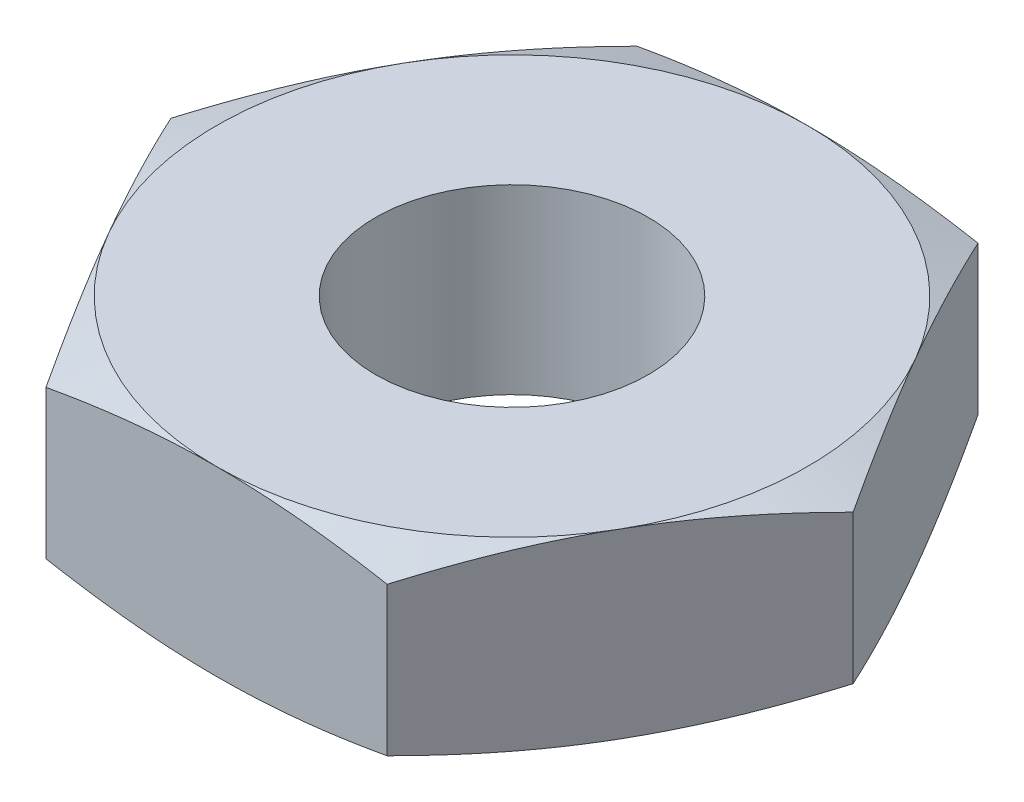
ISO-10303-21;
HEADER;
FILE_DESCRIPTION(('STEP AP214'),'2;1');
FILE_NAME('part.step','',(''),(''),'','','');
FILE_SCHEMA(('AUTOMOTIVE_DESIGN { 1 0 10303 214 1 1 1 1 }'));
ENDSEC;
DATA;
#1=APPLICATION_CONTEXT('core data for automotive mechanical design processes');
#2=APPLICATION_PROTOCOL_DEFINITION('international standard','automotive_design',2000,#1);
#3=PRODUCT_CONTEXT('',#1,'mechanical');
#4=PRODUCT('Part','Part','',(#3));
#5=PRODUCT_RELATED_PRODUCT_CATEGORY('part','',(#4));
#6=PRODUCT_DEFINITION_FORMATION('','',#4);
#7=PRODUCT_DEFINITION_CONTEXT('part definition',#1,'design');
#8=PRODUCT_DEFINITION('design','',#6,#7);
#9=PRODUCT_DEFINITION_SHAPE('','',#8);
#10=(LENGTH_UNIT() NAMED_UNIT(*) SI_UNIT(.MILLI.,.METRE.));
#11=(NAMED_UNIT(*) PLANE_ANGLE_UNIT() SI_UNIT($,.RADIAN.));
#12=(NAMED_UNIT(*) SI_UNIT($,.STERADIAN.) SOLID_ANGLE_UNIT());
#13=UNCERTAINTY_MEASURE_WITH_UNIT(LENGTH_MEASURE(1.E-05),#10,'distance_accuracy_value','');
#14=(GEOMETRIC_REPRESENTATION_CONTEXT(3) GLOBAL_UNCERTAINTY_ASSIGNED_CONTEXT((#13)) GLOBAL_UNIT_ASSIGNED_CONTEXT((#10,
#11,#12)) REPRESENTATION_CONTEXT('',''));
#15=CARTESIAN_POINT('',(0.,0.,0.));
#16=DIRECTION('',(0.,0.,1.));
#17=DIRECTION('',(1.,0.,0.));
#18=AXIS2_PLACEMENT_3D('',#15,#16,#17);
#19=CARTESIAN_POINT('',(0.,-4.,0.));
#20=DIRECTION('',(0.,1.,0.));
#21=DIRECTION('',(0.,0.,1.));
#22=AXIS2_PLACEMENT_3D('',#19,#20,#21);
#23=PLANE('',#22);
#24=CARTESIAN_POINT('',(0.,-4.,0.));
#25=DIRECTION('',(0.,1.,0.));
#26=DIRECTION('',(0.,0.,1.));
#27=AXIS2_PLACEMENT_3D('',#24,#25,#26);
#28=CIRCLE('',#27,6.);
#29=CARTESIAN_POINT('',(0.,-4.,6.));
#30=VERTEX_POINT('',#29);
#31=EDGE_CURVE('E260',#30,#30,#28,.T.);
#32=ORIENTED_EDGE('',*,*,#31,.T.);
#33=EDGE_LOOP('',(#32));
#34=FACE_BOUND('',#33,.T.);
#35=CARTESIAN_POINT('',(0.,-4.,0.));
#36=DIRECTION('',(0.,1.,0.));
#37=DIRECTION('',(0.,0.,1.));
#38=AXIS2_PLACEMENT_3D('',#35,#36,#37);
#39=CIRCLE('',#38,13.);
#40=CARTESIAN_POINT('',(1.35208313886344E-13,-4.,13.));
#41=VERTEX_POINT('',#40);
#42=CARTESIAN_POINT('',(11.2583302491977,-4.,6.49999999999994));
#43=VERTEX_POINT('',#42);
#44=EDGE_CURVE('E145',#41,#43,#39,.T.);
#45=ORIENTED_EDGE('',*,*,#44,.F.);
#46=CARTESIAN_POINT('',(0.,-4.,0.));
#47=DIRECTION('',(0.,1.,0.));
#48=DIRECTION('',(0.,0.,1.));
#49=AXIS2_PLACEMENT_3D('',#46,#47,#48);
#50=CIRCLE('',#49,13.);
#51=CARTESIAN_POINT('',(-11.2583302491977,-4.,6.50000000000009));
#52=VERTEX_POINT('',#51);
#53=EDGE_CURVE('E12',#41,#52,#50,.F.);
#54=ORIENTED_EDGE('',*,*,#53,.T.);
#55=CARTESIAN_POINT('',(-11.2583302491977,-4.,-6.49999999999993));
#56=VERTEX_POINT('',#55);
#57=EDGE_CURVE('E49',#52,#56,#50,.F.);
#58=ORIENTED_EDGE('',*,*,#57,.T.);
#59=CARTESIAN_POINT('',(0.,-4.,-13.));
#60=VERTEX_POINT('',#59);
#61=EDGE_CURVE('E456',#56,#60,#50,.F.);
#62=ORIENTED_EDGE('',*,*,#61,.T.);
#63=CARTESIAN_POINT('',(11.2583302491977,-4.,-6.50000000000002));
#64=VERTEX_POINT('',#63);
#65=EDGE_CURVE('E148',#60,#64,#50,.F.);
#66=ORIENTED_EDGE('',*,*,#65,.T.);
#67=EDGE_CURVE('E51',#64,#43,#50,.F.);
#68=ORIENTED_EDGE('',*,*,#67,.T.);
#69=EDGE_LOOP('',(#45,#54,#58,#62,#66,#68));
#70=FACE_BOUND('',#69,.T.);
#71=ADVANCED_FACE('F41',(#34,#70),#23,.F.);
#72=CARTESIAN_POINT('',(0.,4.,0.));
#73=DIRECTION('',(0.,1.,0.));
#74=DIRECTION('',(0.,0.,1.));
#75=AXIS2_PLACEMENT_3D('',#72,#73,#74);
#76=PLANE('',#75);
#77=CARTESIAN_POINT('',(0.,4.,0.));
#78=DIRECTION('',(0.,1.,0.));
#79=DIRECTION('',(0.,0.,1.));
#80=AXIS2_PLACEMENT_3D('',#77,#78,#79);
#81=CIRCLE('',#80,6.);
#82=CARTESIAN_POINT('',(0.,4.,6.));
#83=VERTEX_POINT('',#82);
#84=EDGE_CURVE('E251',#83,#83,#81,.T.);
#85=ORIENTED_EDGE('',*,*,#84,.F.);
#86=EDGE_LOOP('',(#85));
#87=FACE_BOUND('',#86,.T.);
#88=CARTESIAN_POINT('',(0.,4.,0.));
#89=DIRECTION('',(0.,1.,0.));
#90=DIRECTION('',(0.,0.,1.));
#91=AXIS2_PLACEMENT_3D('',#88,#89,#90);
#92=CIRCLE('',#91,13.);
#93=CARTESIAN_POINT('',(-11.2583302491976,4.,6.50000000000009));
#94=VERTEX_POINT('',#93);
#95=CARTESIAN_POINT('',(1.35308431126191E-13,4.,13.));
#96=VERTEX_POINT('',#95);
#97=EDGE_CURVE('E158',#94,#96,#92,.T.);
#98=ORIENTED_EDGE('',*,*,#97,.T.);
#99=CARTESIAN_POINT('',(11.2583302491978,4.,6.49999999999997));
#100=VERTEX_POINT('',#99);
#101=EDGE_CURVE('E156',#96,#100,#92,.T.);
#102=ORIENTED_EDGE('',*,*,#101,.T.);
#103=CARTESIAN_POINT('',(11.2583302491977,4.,-6.50000000000002));
#104=VERTEX_POINT('',#103);
#105=EDGE_CURVE('E302',#100,#104,#92,.T.);
#106=ORIENTED_EDGE('',*,*,#105,.T.);
#107=CARTESIAN_POINT('',(0.,4.,-13.));
#108=VERTEX_POINT('',#107);
#109=EDGE_CURVE('E308',#104,#108,#92,.T.);
#110=ORIENTED_EDGE('',*,*,#109,.T.);
#111=CARTESIAN_POINT('',(-11.2583302491977,4.,-6.49999999999993));
#112=VERTEX_POINT('',#111);
#113=EDGE_CURVE('E309',#108,#112,#92,.T.);
#114=ORIENTED_EDGE('',*,*,#113,.T.);
#115=EDGE_CURVE('E157',#112,#94,#92,.T.);
#116=ORIENTED_EDGE('',*,*,#115,.T.);
#117=EDGE_LOOP('',(#98,#102,#106,#110,#114,#116));
#118=FACE_BOUND('',#117,.T.);
#119=ADVANCED_FACE('F312',(#87,#118),#76,.T.);
#120=CARTESIAN_POINT('',(7.50555349946529,4.,12.9999999999999));
#121=DIRECTION('',(-0.866025403784441,0.,-0.499999999999995));
#122=DIRECTION('',(-0.499999999999995,0.,0.866025403784442));
#123=AXIS2_PLACEMENT_3D('',#120,#121,#122);
#124=PLANE('',#123);
#125=DIRECTION('',(0.,-1.,0.));
#126=VECTOR('',#125,1.);
#127=CARTESIAN_POINT('',(7.50555349946529,4.,12.9999999999999));
#128=LINE('',#127,#126);
#129=CARTESIAN_POINT('',(7.50555349946529,3.26801691446495,12.9999999999999));
#130=VERTEX_POINT('',#129);
#131=CARTESIAN_POINT('',(7.50555349946529,-3.26801691446495,12.9999999999999));
#132=VERTEX_POINT('',#131);
#133=EDGE_CURVE('E153',#130,#132,#128,.T.);
#134=ORIENTED_EDGE('',*,*,#133,.T.);
#135=CARTESIAN_POINT('',(7.50543802941145,-3.26797488631748,13.0001999999999));
#136=CARTESIAN_POINT('',(7.81626903778432,-3.3811479316258,12.4618249009302));
#137=CARTESIAN_POINT('',(8.12812500165726,-3.48409821469969,11.9216745268589));
#138=CARTESIAN_POINT('',(8.75386455582981,-3.66522307853089,10.8378618267266));
#139=CARTESIAN_POINT('',(9.06774953779601,-3.7433782740141,10.2941970902283));
#140=CARTESIAN_POINT('',(9.69406389084071,-3.86979198052381,9.20938880924519));
#141=CARTESIAN_POINT('',(10.0064789597828,-3.91832620674503,8.66827003678739));
#142=CARTESIAN_POINT('',(10.6320396475706,-3.98342422307978,7.58476714232116));
#143=CARTESIAN_POINT('',(10.9451849483842,-3.99999999999998,7.04238357116056));
#144=CARTESIAN_POINT('',(11.5714755500114,-3.99999999999998,5.95761642883936));
#145=CARTESIAN_POINT('',(11.884620850825,-3.98342422307978,5.41523285767877));
#146=CARTESIAN_POINT('',(12.5101815386128,-3.91832620674503,4.33172996321253));
#147=CARTESIAN_POINT('',(12.8225966075549,-3.8697919805238,3.79061119075473));
#148=CARTESIAN_POINT('',(13.4489109605996,-3.7433782740141,2.70580290977165));
#149=CARTESIAN_POINT('',(13.7627959425658,-3.66522307853089,2.16213817327336));
#150=CARTESIAN_POINT('',(14.3885354967383,-3.48409821469969,1.07832547314098));
#151=CARTESIAN_POINT('',(14.7003914606113,-3.3811479316258,0.538175099069677));
#152=CARTESIAN_POINT('',(15.0112224689841,-3.26797488631748,-0.000199999999997858));
#153=B_SPLINE_CURVE_WITH_KNOTS('',3,(#135,#136,#137,#138,#139,#140,#141,#142,#143,#144,#145,
#146,#147,#148,#149,#150,#151,#152),.UNSPECIFIED.,.F.,.F.,(4,2,2,2,2,2,2,2,4),(0.,
1.89583425179581,3.79314707118518,5.67251886941189,7.5511856255365,9.4298523816611,
11.3092241798878,13.2065369992772,15.102371251073),.UNSPECIFIED.);
#154=EDGE_CURVE('E64',#132,#43,#153,.T.);
#155=ORIENTED_EDGE('',*,*,#154,.T.);
#156=CARTESIAN_POINT('',(15.0111069989303,-3.26801691446495,0.));
#157=VERTEX_POINT('',#156);
#158=EDGE_CURVE('E132',#43,#157,#153,.T.);
#159=ORIENTED_EDGE('',*,*,#158,.T.);
#160=DIRECTION('',(0.,-1.,0.));
#161=VECTOR('',#160,1.);
#162=CARTESIAN_POINT('',(15.0111069989303,4.,0.));
#163=LINE('',#162,#161);
#164=CARTESIAN_POINT('',(15.0111069989303,3.26801691446495,0.));
#165=VERTEX_POINT('',#164);
#166=EDGE_CURVE('E271',#165,#157,#163,.T.);
#167=ORIENTED_EDGE('',*,*,#166,.F.);
#168=CARTESIAN_POINT('',(7.50543802941145,3.26797488631748,13.0001999999999));
#169=CARTESIAN_POINT('',(7.81626903778432,3.3811479316258,12.4618249009302));
#170=CARTESIAN_POINT('',(8.12812500165726,3.48409821469969,11.9216745268589));
#171=CARTESIAN_POINT('',(8.75386455582981,3.66522307853089,10.8378618267266));
#172=CARTESIAN_POINT('',(9.06774953779601,3.7433782740141,10.2941970902283));
#173=CARTESIAN_POINT('',(9.69406389084071,3.86979198052381,9.20938880924519));
#174=CARTESIAN_POINT('',(10.0064789597828,3.91832620674503,8.66827003678739));
#175=CARTESIAN_POINT('',(10.6320396475706,3.98342422307978,7.58476714232116));
#176=CARTESIAN_POINT('',(10.9451849483842,3.99999999999998,7.04238357116056));
#177=CARTESIAN_POINT('',(11.5714755500114,3.99999999999998,5.95761642883936));
#178=CARTESIAN_POINT('',(11.884620850825,3.98342422307978,5.41523285767877));
#179=CARTESIAN_POINT('',(12.5101815386128,3.91832620674503,4.33172996321253));
#180=CARTESIAN_POINT('',(12.8225966075549,3.8697919805238,3.79061119075473));
#181=CARTESIAN_POINT('',(13.4489109605996,3.7433782740141,2.70580290977165));
#182=CARTESIAN_POINT('',(13.7627959425658,3.66522307853089,2.16213817327336));
#183=CARTESIAN_POINT('',(14.3885354967383,3.48409821469969,1.07832547314098));
#184=CARTESIAN_POINT('',(14.7003914606113,3.3811479316258,0.538175099069677));
#185=CARTESIAN_POINT('',(15.0112224689841,3.26797488631748,-0.000199999999997858));
#186=B_SPLINE_CURVE_WITH_KNOTS('',3,(#168,#169,#170,#171,#172,#173,#174,#175,#176,#177,#178,
#179,#180,#181,#182,#183,#184,#185),.UNSPECIFIED.,.F.,.F.,(4,2,2,2,2,2,2,2,4),(0.,
1.89583425179581,3.79314707118518,5.67251886941189,7.5511856255365,9.4298523816611,
11.3092241798878,13.2065369992772,15.102371251073),.UNSPECIFIED.);
#187=EDGE_CURVE('E250',#100,#165,#186,.T.);
#188=ORIENTED_EDGE('',*,*,#187,.F.);
#189=EDGE_CURVE('E254',#130,#100,#186,.T.);
#190=ORIENTED_EDGE('',*,*,#189,.F.);
#191=EDGE_LOOP('',(#134,#155,#159,#167,#188,#190));
#192=FACE_BOUND('',#191,.T.);
#193=ADVANCED_FACE('F43',(#192),#124,.F.);
#194=CARTESIAN_POINT('',(15.0111069989303,4.,0.));
#195=DIRECTION('',(-0.866025403784438,0.,0.500000000000001));
#196=DIRECTION('',(0.500000000000001,0.,0.866025403784438));
#197=AXIS2_PLACEMENT_3D('',#194,#195,#196);
#198=PLANE('',#197);
#199=ORIENTED_EDGE('',*,*,#166,.T.);
#200=CARTESIAN_POINT('',(15.0112224689841,-3.26797488631748,0.000200000000000042));
#201=CARTESIAN_POINT('',(14.7003914606112,-3.38114793162581,-0.53817509906968));
#202=CARTESIAN_POINT('',(14.3885354967383,-3.48409821469969,-1.07832547314099));
#203=CARTESIAN_POINT('',(13.7627959425657,-3.6652230785309,-2.16213817327337));
#204=CARTESIAN_POINT('',(13.4489109605995,-3.74337827401411,-2.70580290977167));
#205=CARTESIAN_POINT('',(12.8225966075548,-3.86979198052382,-3.79061119075476));
#206=CARTESIAN_POINT('',(12.5101815386127,-3.91832620674505,-4.33172996321257));
#207=CARTESIAN_POINT('',(11.8846208508249,-3.9834242230798,-5.41523285767881));
#208=CARTESIAN_POINT('',(11.5714755500113,-4.,-5.95761642883941));
#209=CARTESIAN_POINT('',(10.9451849483841,-4.,-7.04238357116062));
#210=CARTESIAN_POINT('',(10.6320396475705,-3.9834242230798,-7.58476714232122));
#211=CARTESIAN_POINT('',(10.0064789597827,-3.91832620674505,-8.66827003678746));
#212=CARTESIAN_POINT('',(9.69406389084059,-3.86979198052382,-9.20938880924526));
#213=CARTESIAN_POINT('',(9.06774953779586,-3.74337827401411,-10.2941970902284));
#214=CARTESIAN_POINT('',(8.75386455582966,-3.6652230785309,-10.8378618267267));
#215=CARTESIAN_POINT('',(8.12812500165709,-3.48409821469969,-11.921674526859));
#216=CARTESIAN_POINT('',(7.81626903778414,-3.38114793162581,-12.4618249009303));
#217=CARTESIAN_POINT('',(7.50543802941127,-3.26797488631748,-13.0002));
#218=B_SPLINE_CURVE_WITH_KNOTS('',3,(#200,#201,#202,#203,#204,#205,#206,#207,#208,#209,#210,
#211,#212,#213,#214,#215,#216,#217),.UNSPECIFIED.,.F.,.F.,(4,2,2,2,2,2,2,2,4),(0.,
1.89583425179583,3.79314707118523,5.67251886941196,7.55118562553659,9.42985238166122,
11.309224179888,13.2065369992774,15.1023712510732),.UNSPECIFIED.);
#219=EDGE_CURVE('E138',#157,#64,#218,.T.);
#220=ORIENTED_EDGE('',*,*,#219,.T.);
#221=CARTESIAN_POINT('',(7.50555349946511,-3.26801691446495,-13.));
#222=VERTEX_POINT('',#221);
#223=EDGE_CURVE('E170',#64,#222,#218,.T.);
#224=ORIENTED_EDGE('',*,*,#223,.T.);
#225=DIRECTION('',(0.,-1.,0.));
#226=VECTOR('',#225,1.);
#227=CARTESIAN_POINT('',(7.50555349946511,4.,-13.));
#228=LINE('',#227,#226);
#229=CARTESIAN_POINT('',(7.50555349946511,3.26801691446495,-13.));
#230=VERTEX_POINT('',#229);
#231=EDGE_CURVE('E266',#230,#222,#228,.T.);
#232=ORIENTED_EDGE('',*,*,#231,.F.);
#233=CARTESIAN_POINT('',(15.0112224689841,3.26797488631748,0.000200000000000042));
#234=CARTESIAN_POINT('',(14.7003914606112,3.38114793162581,-0.53817509906968));
#235=CARTESIAN_POINT('',(14.3885354967383,3.48409821469969,-1.07832547314099));
#236=CARTESIAN_POINT('',(13.7627959425657,3.6652230785309,-2.16213817327337));
#237=CARTESIAN_POINT('',(13.4489109605995,3.74337827401411,-2.70580290977167));
#238=CARTESIAN_POINT('',(12.8225966075548,3.86979198052382,-3.79061119075476));
#239=CARTESIAN_POINT('',(12.5101815386127,3.91832620674505,-4.33172996321257));
#240=CARTESIAN_POINT('',(11.8846208508249,3.9834242230798,-5.41523285767881));
#241=CARTESIAN_POINT('',(11.5714755500113,4.,-5.95761642883941));
#242=CARTESIAN_POINT('',(10.9451849483841,4.,-7.04238357116062));
#243=CARTESIAN_POINT('',(10.6320396475705,3.9834242230798,-7.58476714232122));
#244=CARTESIAN_POINT('',(10.0064789597827,3.91832620674505,-8.66827003678746));
#245=CARTESIAN_POINT('',(9.69406389084059,3.86979198052382,-9.20938880924526));
#246=CARTESIAN_POINT('',(9.06774953779586,3.74337827401411,-10.2941970902284));
#247=CARTESIAN_POINT('',(8.75386455582966,3.6652230785309,-10.8378618267267));
#248=CARTESIAN_POINT('',(8.12812500165709,3.48409821469969,-11.921674526859));
#249=CARTESIAN_POINT('',(7.81626903778414,3.38114793162581,-12.4618249009303));
#250=CARTESIAN_POINT('',(7.50543802941127,3.26797488631748,-13.0002));
#251=B_SPLINE_CURVE_WITH_KNOTS('',3,(#233,#234,#235,#236,#237,#238,#239,#240,#241,#242,#243,
#244,#245,#246,#247,#248,#249,#250),.UNSPECIFIED.,.F.,.F.,(4,2,2,2,2,2,2,2,4),(0.,
1.89583425179583,3.79314707118523,5.67251886941196,7.55118562553659,9.42985238166122,
11.309224179888,13.2065369992774,15.1023712510732),.UNSPECIFIED.);
#252=EDGE_CURVE('E239',#104,#230,#251,.T.);
#253=ORIENTED_EDGE('',*,*,#252,.F.);
#254=EDGE_CURVE('E246',#165,#104,#251,.T.);
#255=ORIENTED_EDGE('',*,*,#254,.F.);
#256=EDGE_LOOP('',(#199,#220,#224,#232,#253,#255));
#257=FACE_BOUND('',#256,.T.);
#258=ADVANCED_FACE('F218',(#257),#198,.F.);
#259=CARTESIAN_POINT('',(7.50555349946511,4.,-13.));
#260=DIRECTION('',(0.,0.,1.));
#261=DIRECTION('',(1.,0.,0.));
#262=AXIS2_PLACEMENT_3D('',#259,#260,#261);
#263=PLANE('',#262);
#264=ORIENTED_EDGE('',*,*,#231,.T.);
#265=CARTESIAN_POINT('',(24.5155545956959,1.36823250554055,-13.0000000000001));
#266=CARTESIAN_POINT('',(24.0405240295999,1.21549334301211,-13.0000000000001));
#267=CARTESIAN_POINT('',(23.5652140208819,1.063618435089,-13.0000000000001));
#268=CARTESIAN_POINT('',(22.6139411221326,0.761910318310484,-13.0000000000001));
#269=CARTESIAN_POINT('',(22.1379782252003,0.612077131221862,-13.0000000000001));
#270=CARTESIAN_POINT('',(21.185215660392,0.314737702143928,-13.0000000000001));
#271=CARTESIAN_POINT('',(20.7084158378096,0.167231955324839,-13.0000000000001));
#272=CARTESIAN_POINT('',(19.7539723799837,-0.125022680870063,-13.0000000000001));
#273=CARTESIAN_POINT('',(19.2763287466556,-0.269771576494738,-13.0000000000001));
#274=CARTESIAN_POINT('',(18.3122096400441,-0.558389376293444,-13.0000000000001));
#275=CARTESIAN_POINT('',(17.8257180947263,-0.70220466785382,-13.0000000000001));
#276=CARTESIAN_POINT('',(16.8515839809399,-0.985880989376546,-13.0000000000001));
#277=CARTESIAN_POINT('',(16.3639414177948,-1.12574203758895,-13.0000000000001));
#278=CARTESIAN_POINT('',(15.3873473631516,-1.40075431206701,-13.0000000000001));
#279=CARTESIAN_POINT('',(14.8983959224935,-1.53590571848869,-13.));
#280=CARTESIAN_POINT('',(13.9189691583564,-1.80058323746787,-13.));
#281=CARTESIAN_POINT('',(13.428493836208,-1.93010935493618,-13.));
#282=CARTESIAN_POINT('',(12.4681215109835,-2.17667647391496,-13.));
#283=CARTESIAN_POINT('',(11.9983017482554,-2.29401734212416,-13.));
#284=CARTESIAN_POINT('',(11.0568829216087,-2.52135287481595,-13.));
#285=CARTESIAN_POINT('',(10.5852838557062,-2.63134753110473,-13.));
#286=CARTESIAN_POINT('',(9.64003084776995,-2.84258990322838,-13.));
#287=CARTESIAN_POINT('',(9.16637658007017,-2.9438361753631,-13.));
#288=CARTESIAN_POINT('',(8.21697677002227,-3.13589877665886,-13.));
#289=CARTESIAN_POINT('',(7.74123122545284,-3.22671509473869,-13.));
#290=CARTESIAN_POINT('',(6.31910363449161,-3.47919521660132,-13.));
#291=CARTESIAN_POINT('',(5.36932395191108,-3.62285615701864,-13.));
#292=CARTESIAN_POINT('',(3.93925896632588,-3.79026925410424,-13.));
#293=CARTESIAN_POINT('',(3.46174282400493,-3.83805703289572,-13.));
#294=CARTESIAN_POINT('',(2.50523859716394,-3.91592711867877,-13.));
#295=CARTESIAN_POINT('',(2.02625050436415,-3.9460093258922,-13.));
#296=CARTESIAN_POINT('',(1.00608586276806,-3.98987319438264,-13.));
#297=CARTESIAN_POINT('',(0.464795352583161,-4.00107614649847,-13.));
#298=CARTESIAN_POINT('',(-0.617736217142298,-3.99876013196134,-13.));
#299=CARTESIAN_POINT('',(-1.15897727593229,-3.98524083761707,-13.));
#300=CARTESIAN_POINT('',(-2.24052002292679,-3.93421249506995,-13.));
#301=CARTESIAN_POINT('',(-2.78082126229037,-3.89669409003737,-13.));
#302=CARTESIAN_POINT('',(-3.85941505627078,-3.79955682519537,-13.));
#303=CARTESIAN_POINT('',(-4.39770756186364,-3.73993742951957,-13.));
#304=CARTESIAN_POINT('',(-5.47704146456944,-3.60052693841533,-13.));
#305=CARTESIAN_POINT('',(-6.01805758084636,-3.5205426199044,-13.));
#306=CARTESIAN_POINT('',(-7.09728629812356,-3.34363373953174,-13.));
#307=CARTESIAN_POINT('',(-7.63549887790093,-3.24670904962198,-13.));
#308=CARTESIAN_POINT('',(-8.70920964168745,-3.03872213356502,-13.));
#309=CARTESIAN_POINT('',(-9.24470758968157,-2.92765869936841,-13.));
#310=CARTESIAN_POINT('',(-10.3131373904122,-2.6938904888945,-13.));
#311=CARTESIAN_POINT('',(-10.8460692509991,-2.57118574825494,-13.));
#312=CARTESIAN_POINT('',(-11.9378787322153,-2.30946863118862,-13.));
#313=CARTESIAN_POINT('',(-12.496631109914,-2.16993626646767,-13.));
#314=CARTESIAN_POINT('',(-13.61191651028,-1.88230159824707,-13.));
#315=CARTESIAN_POINT('',(-14.1684495289799,-1.73419927943467,-13.));
#316=CARTESIAN_POINT('',(-15.2795521826457,-1.43104180462645,-12.9999999999999));
#317=CARTESIAN_POINT('',(-15.83412201007,-1.27598735175158,-12.9999999999999));
#318=CARTESIAN_POINT('',(-16.941638337672,-0.960181887271385,-12.9999999999999));
#319=CARTESIAN_POINT('',(-17.4945848238111,-0.799430826558432,-12.9999999999999));
#320=CARTESIAN_POINT('',(-18.5881502472213,-0.476472370913964,-12.9999999999999));
#321=CARTESIAN_POINT('',(-19.128796391371,-0.314356915140173,-12.9999999999999));
#322=CARTESIAN_POINT('',(-20.2089506297819,0.0136235671370092,-12.9999999999999));
#323=CARTESIAN_POINT('',(-20.748458720098,0.179488606615906,-12.9999999999999));
#324=CARTESIAN_POINT('',(-21.8263834446703,0.514319692132321,-12.9999999999999));
#325=CARTESIAN_POINT('',(-22.3648002881825,0.683285065514164,-12.9999999999999));
#326=CARTESIAN_POINT('',(-23.4407814868745,1.02387855364092,-12.9999999999999));
#327=CARTESIAN_POINT('',(-23.9783458563606,1.19550662316754,-12.9999999999999));
#328=CARTESIAN_POINT('',(-24.515554595696,1.36823250554055,-12.9999999999999));
#329=B_SPLINE_CURVE_WITH_KNOTS('',3,(#265,#266,#267,#268,#269,#270,#271,#272,#273,#274,#275,
#276,#277,#278,#279,#280,#281,#282,#283,#284,#285,#286,#287,#288,#289,#290,#291,#292,#293,#294,
#295,#296,#297,#298,#299,#300,#301,#302,#303,#304,#305,#306,#307,#308,#309,#310,#311,#312,#313,
#314,#315,#316,#317,#318,#319,#320,#321,#322,#323,#324,#325,#326,#327,#328),.UNSPECIFIED.,.F.,
.F.,(4,2,2,2,2,2,2,2,2,2,2,2,2,2,2,2,2,2,2,2,2,2,2,2,2,2,2,2,2,2,2,4),(0.,1.49694813967669,
2.99391222584255,4.49119061440192,5.98846560872694,7.51036210879345,9.03225158369156,
10.5540827783197,12.0759126443824,13.5286166449153,14.9813222657356,16.4342671629383,
17.8872136037934,20.7669364113332,22.2063696578436,23.6458110160719,25.2694632279234,
26.893136961305,28.5174441225877,30.1417906698226,31.7821640738609,33.4225498776076,
35.063075934178,36.7035969687382,38.4312458729983,40.1588978643094,41.8863755177535,
43.6138680665518,45.3071379597887,47.0004137135154,48.6933263352441,50.3862102390845),.UNSPECIFIED.);
#330=EDGE_CURVE('E211',#222,#60,#329,.T.);
#331=ORIENTED_EDGE('',*,*,#330,.T.);
#332=CARTESIAN_POINT('',(-7.5055534994652,-3.26801691446495,-13.));
#333=VERTEX_POINT('',#332);
#334=EDGE_CURVE('E210',#60,#333,#329,.T.);
#335=ORIENTED_EDGE('',*,*,#334,.T.);
#336=DIRECTION('',(0.,-1.,0.));
#337=VECTOR('',#336,1.);
#338=CARTESIAN_POINT('',(-7.5055534994652,4.,-13.));
#339=LINE('',#338,#337);
#340=CARTESIAN_POINT('',(-7.5055534994652,3.26801691446495,-13.));
#341=VERTEX_POINT('',#340);
#342=EDGE_CURVE('E269',#341,#333,#339,.T.);
#343=ORIENTED_EDGE('',*,*,#342,.F.);
#344=CARTESIAN_POINT('',(24.5155545956959,-1.36823250554055,-13.0000000000001));
#345=CARTESIAN_POINT('',(24.0405240295999,-1.21549334301211,-13.0000000000001));
#346=CARTESIAN_POINT('',(23.5652140208819,-1.063618435089,-13.0000000000001));
#347=CARTESIAN_POINT('',(22.6139411221326,-0.761910318310484,-13.0000000000001));
#348=CARTESIAN_POINT('',(22.1379782252003,-0.612077131221862,-13.0000000000001));
#349=CARTESIAN_POINT('',(21.185215660392,-0.314737702143928,-13.0000000000001));
#350=CARTESIAN_POINT('',(20.7084158378096,-0.167231955324839,-13.0000000000001));
#351=CARTESIAN_POINT('',(19.7539723799837,0.125022680870063,-13.0000000000001));
#352=CARTESIAN_POINT('',(19.2763287466556,0.269771576494738,-13.0000000000001));
#353=CARTESIAN_POINT('',(18.3122096400441,0.558389376293444,-13.0000000000001));
#354=CARTESIAN_POINT('',(17.8257180947263,0.70220466785382,-13.0000000000001));
#355=CARTESIAN_POINT('',(16.8515839809399,0.985880989376546,-13.0000000000001));
#356=CARTESIAN_POINT('',(16.3639414177948,1.12574203758895,-13.0000000000001));
#357=CARTESIAN_POINT('',(15.3873473631516,1.40075431206701,-13.0000000000001));
#358=CARTESIAN_POINT('',(14.8983959224935,1.53590571848869,-13.));
#359=CARTESIAN_POINT('',(13.9189691583564,1.80058323746787,-13.));
#360=CARTESIAN_POINT('',(13.428493836208,1.93010935493618,-13.));
#361=CARTESIAN_POINT('',(12.4681215109835,2.17667647391496,-13.));
#362=CARTESIAN_POINT('',(11.9983017482554,2.29401734212416,-13.));
#363=CARTESIAN_POINT('',(11.0568829216087,2.52135287481595,-13.));
#364=CARTESIAN_POINT('',(10.5852838557062,2.63134753110473,-13.));
#365=CARTESIAN_POINT('',(9.64003084776995,2.84258990322838,-13.));
#366=CARTESIAN_POINT('',(9.16637658007017,2.9438361753631,-13.));
#367=CARTESIAN_POINT('',(8.21697677002227,3.13589877665886,-13.));
#368=CARTESIAN_POINT('',(7.74123122545284,3.22671509473869,-13.));
#369=CARTESIAN_POINT('',(6.31910363449161,3.47919521660132,-13.));
#370=CARTESIAN_POINT('',(5.36932395191108,3.62285615701864,-13.));
#371=CARTESIAN_POINT('',(3.93925896632588,3.79026925410424,-13.));
#372=CARTESIAN_POINT('',(3.46174282400493,3.83805703289572,-13.));
#373=CARTESIAN_POINT('',(2.50523859716394,3.91592711867877,-13.));
#374=CARTESIAN_POINT('',(2.02625050436415,3.9460093258922,-13.));
#375=CARTESIAN_POINT('',(1.00608586276806,3.98987319438264,-13.));
#376=CARTESIAN_POINT('',(0.464795352583161,4.00107614649847,-13.));
#377=CARTESIAN_POINT('',(-0.617736217142298,3.99876013196134,-13.));
#378=CARTESIAN_POINT('',(-1.15897727593229,3.98524083761707,-13.));
#379=CARTESIAN_POINT('',(-2.24052002292679,3.93421249506995,-13.));
#380=CARTESIAN_POINT('',(-2.78082126229037,3.89669409003737,-13.));
#381=CARTESIAN_POINT('',(-3.85941505627078,3.79955682519537,-13.));
#382=CARTESIAN_POINT('',(-4.39770756186364,3.73993742951957,-13.));
#383=CARTESIAN_POINT('',(-5.47704146456944,3.60052693841533,-13.));
#384=CARTESIAN_POINT('',(-6.01805758084636,3.5205426199044,-13.));
#385=CARTESIAN_POINT('',(-7.09728629812356,3.34363373953174,-13.));
#386=CARTESIAN_POINT('',(-7.63549887790093,3.24670904962198,-13.));
#387=CARTESIAN_POINT('',(-8.70920964168745,3.03872213356502,-13.));
#388=CARTESIAN_POINT('',(-9.24470758968157,2.92765869936841,-13.));
#389=CARTESIAN_POINT('',(-10.3131373904122,2.6938904888945,-13.));
#390=CARTESIAN_POINT('',(-10.8460692509991,2.57118574825494,-13.));
#391=CARTESIAN_POINT('',(-11.9378787322153,2.30946863118862,-13.));
#392=CARTESIAN_POINT('',(-12.496631109914,2.16993626646767,-13.));
#393=CARTESIAN_POINT('',(-13.61191651028,1.88230159824707,-13.));
#394=CARTESIAN_POINT('',(-14.1684495289799,1.73419927943467,-13.));
#395=CARTESIAN_POINT('',(-15.2795521826457,1.43104180462645,-12.9999999999999));
#396=CARTESIAN_POINT('',(-15.83412201007,1.27598735175158,-12.9999999999999));
#397=CARTESIAN_POINT('',(-16.941638337672,0.960181887271385,-12.9999999999999));
#398=CARTESIAN_POINT('',(-17.4945848238111,0.799430826558432,-12.9999999999999));
#399=CARTESIAN_POINT('',(-18.5881502472213,0.476472370913964,-12.9999999999999));
#400=CARTESIAN_POINT('',(-19.128796391371,0.314356915140173,-12.9999999999999));
#401=CARTESIAN_POINT('',(-20.2089506297819,-0.0136235671370092,-12.9999999999999));
#402=CARTESIAN_POINT('',(-20.748458720098,-0.179488606615906,-12.9999999999999));
#403=CARTESIAN_POINT('',(-21.8263834446703,-0.514319692132321,-12.9999999999999));
#404=CARTESIAN_POINT('',(-22.3648002881825,-0.683285065514164,-12.9999999999999));
#405=CARTESIAN_POINT('',(-23.4407814868745,-1.02387855364092,-12.9999999999999));
#406=CARTESIAN_POINT('',(-23.9783458563606,-1.19550662316754,-12.9999999999999));
#407=CARTESIAN_POINT('',(-24.515554595696,-1.36823250554055,-12.9999999999999));
#408=B_SPLINE_CURVE_WITH_KNOTS('',3,(#344,#345,#346,#347,#348,#349,#350,#351,#352,#353,#354,
#355,#356,#357,#358,#359,#360,#361,#362,#363,#364,#365,#366,#367,#368,#369,#370,#371,#372,#373,
#374,#375,#376,#377,#378,#379,#380,#381,#382,#383,#384,#385,#386,#387,#388,#389,#390,#391,#392,
#393,#394,#395,#396,#397,#398,#399,#400,#401,#402,#403,#404,#405,#406,#407),.UNSPECIFIED.,.F.,
.F.,(4,2,2,2,2,2,2,2,2,2,2,2,2,2,2,2,2,2,2,2,2,2,2,2,2,2,2,2,2,2,2,4),(0.,1.49694813967669,
2.99391222584255,4.49119061440192,5.98846560872694,7.51036210879345,9.03225158369156,
10.5540827783197,12.0759126443824,13.5286166449153,14.9813222657356,16.4342671629383,
17.8872136037934,20.7669364113332,22.2063696578436,23.6458110160719,25.2694632279234,
26.893136961305,28.5174441225877,30.1417906698226,31.7821640738609,33.4225498776076,
35.063075934178,36.7035969687382,38.4312458729983,40.1588978643094,41.8863755177535,
43.6138680665518,45.3071379597887,47.0004137135154,48.6933263352441,50.3862102390845),.UNSPECIFIED.);
#409=EDGE_CURVE('E228',#108,#341,#408,.T.);
#410=ORIENTED_EDGE('',*,*,#409,.F.);
#411=EDGE_CURVE('E231',#230,#108,#408,.T.);
#412=ORIENTED_EDGE('',*,*,#411,.F.);
#413=EDGE_LOOP('',(#264,#331,#335,#343,#410,#412));
#414=FACE_BOUND('',#413,.T.);
#415=ADVANCED_FACE('F217',(#414),#263,.F.);
#416=CARTESIAN_POINT('',(-7.5055534994652,4.,-13.));
#417=DIRECTION('',(0.866025403784442,0.,0.499999999999995));
#418=DIRECTION('',(0.499999999999995,0.,-0.866025403784442));
#419=AXIS2_PLACEMENT_3D('',#416,#417,#418);
#420=PLANE('',#419);
#421=ORIENTED_EDGE('',*,*,#342,.T.);
#422=CARTESIAN_POINT('',(-7.50543802941136,-3.26797488631748,-13.0002));
#423=CARTESIAN_POINT('',(-7.81626903778423,-3.38114793162581,-12.4618249009303));
#424=CARTESIAN_POINT('',(-8.12812500165717,-3.48409821469969,-11.921674526859));
#425=CARTESIAN_POINT('',(-8.75386455582973,-3.6652230785309,-10.8378618267266));
#426=CARTESIAN_POINT('',(-9.06774953779593,-3.74337827401411,-10.2941970902283));
#427=CARTESIAN_POINT('',(-9.69406389084065,-3.86979198052382,-9.2093888092452));
#428=CARTESIAN_POINT('',(-10.0064789597827,-3.91832620674505,-8.66827003678739));
#429=CARTESIAN_POINT('',(-10.6320396475705,-3.9834242230798,-7.58476714232115));
#430=CARTESIAN_POINT('',(-10.9451849483841,-4.,-7.04238357116054));
#431=CARTESIAN_POINT('',(-11.5714755500113,-4.,-5.95761642883933));
#432=CARTESIAN_POINT('',(-11.8846208508249,-3.9834242230798,-5.41523285767873));
#433=CARTESIAN_POINT('',(-12.5101815386128,-3.91832620674505,-4.33172996321248));
#434=CARTESIAN_POINT('',(-12.8225966075548,-3.86979198052382,-3.79061119075468));
#435=CARTESIAN_POINT('',(-13.4489109605995,-3.74337827401411,-2.70580290977158));
#436=CARTESIAN_POINT('',(-13.7627959425657,-3.6652230785309,-2.16213817327328));
#437=CARTESIAN_POINT('',(-14.3885354967383,-3.4840982146997,-1.07832547314089));
#438=CARTESIAN_POINT('',(-14.7003914606112,-3.38114793162581,-0.538175099069577));
#439=CARTESIAN_POINT('',(-15.0112224689841,-3.26797488631748,0.000200000000103726));
#440=B_SPLINE_CURVE_WITH_KNOTS('',3,(#422,#423,#424,#425,#426,#427,#428,#429,#430,#431,#432,
#433,#434,#435,#436,#437,#438,#439),.UNSPECIFIED.,.F.,.F.,(4,2,2,2,2,2,2,2,4),(0.,
1.89583425179583,3.79314707118523,5.67251886941196,7.55118562553659,9.42985238166122,
11.3092241798879,13.2065369992773,15.1023712510732),.UNSPECIFIED.);
#441=EDGE_CURVE('E213',#333,#56,#440,.T.);
#442=ORIENTED_EDGE('',*,*,#441,.T.);
#443=CARTESIAN_POINT('',(-15.0111069989303,-3.26801691446495,1.04808663662242E-13));
#444=VERTEX_POINT('',#443);
#445=EDGE_CURVE('E203',#56,#444,#440,.T.);
#446=ORIENTED_EDGE('',*,*,#445,.T.);
#447=DIRECTION('',(0.,-1.,0.));
#448=VECTOR('',#447,1.);
#449=CARTESIAN_POINT('',(-15.0111069989303,4.,1.04821999924285E-13));
#450=LINE('',#449,#448);
#451=CARTESIAN_POINT('',(-15.0111069989303,3.26801691446495,1.04808663662242E-13));
#452=VERTEX_POINT('',#451);
#453=EDGE_CURVE('E261',#452,#444,#450,.T.);
#454=ORIENTED_EDGE('',*,*,#453,.F.);
#455=CARTESIAN_POINT('',(-7.50543802941136,3.26797488631748,-13.0002));
#456=CARTESIAN_POINT('',(-7.81626903778423,3.38114793162581,-12.4618249009303));
#457=CARTESIAN_POINT('',(-8.12812500165717,3.48409821469969,-11.921674526859));
#458=CARTESIAN_POINT('',(-8.75386455582973,3.6652230785309,-10.8378618267266));
#459=CARTESIAN_POINT('',(-9.06774953779593,3.74337827401411,-10.2941970902283));
#460=CARTESIAN_POINT('',(-9.69406389084065,3.86979198052382,-9.2093888092452));
#461=CARTESIAN_POINT('',(-10.0064789597827,3.91832620674505,-8.66827003678739));
#462=CARTESIAN_POINT('',(-10.6320396475705,3.9834242230798,-7.58476714232115));
#463=CARTESIAN_POINT('',(-10.9451849483841,4.,-7.04238357116054));
#464=CARTESIAN_POINT('',(-11.5714755500113,4.,-5.95761642883933));
#465=CARTESIAN_POINT('',(-11.8846208508249,3.9834242230798,-5.41523285767873));
#466=CARTESIAN_POINT('',(-12.5101815386128,3.91832620674505,-4.33172996321248));
#467=CARTESIAN_POINT('',(-12.8225966075548,3.86979198052382,-3.79061119075468));
#468=CARTESIAN_POINT('',(-13.4489109605995,3.74337827401411,-2.70580290977158));
#469=CARTESIAN_POINT('',(-13.7627959425657,3.6652230785309,-2.16213817327328));
#470=CARTESIAN_POINT('',(-14.3885354967383,3.4840982146997,-1.07832547314089));
#471=CARTESIAN_POINT('',(-14.7003914606112,3.38114793162581,-0.538175099069577));
#472=CARTESIAN_POINT('',(-15.0112224689841,3.26797488631748,0.000200000000103726));
#473=B_SPLINE_CURVE_WITH_KNOTS('',3,(#455,#456,#457,#458,#459,#460,#461,#462,#463,#464,#465,
#466,#467,#468,#469,#470,#471,#472),.UNSPECIFIED.,.F.,.F.,(4,2,2,2,2,2,2,2,4),(0.,
1.89583425179583,3.79314707118523,5.67251886941196,7.55118562553659,9.42985238166122,
11.3092241798879,13.2065369992773,15.1023712510732),.UNSPECIFIED.);
#474=EDGE_CURVE('E232',#112,#452,#473,.T.);
#475=ORIENTED_EDGE('',*,*,#474,.F.);
#476=EDGE_CURVE('E234',#341,#112,#473,.T.);
#477=ORIENTED_EDGE('',*,*,#476,.F.);
#478=EDGE_LOOP('',(#421,#442,#446,#454,#475,#477));
#479=FACE_BOUND('',#478,.T.);
#480=ADVANCED_FACE('F216',(#479),#420,.F.);
#481=CARTESIAN_POINT('',(-15.0111069989303,4.,1.04821999924285E-13));
#482=DIRECTION('',(0.866025403784435,0.,-0.500000000000007));
#483=DIRECTION('',(-0.500000000000007,0.,-0.866025403784435));
#484=AXIS2_PLACEMENT_3D('',#481,#482,#483);
#485=PLANE('',#484);
#486=ORIENTED_EDGE('',*,*,#453,.T.);
#487=CARTESIAN_POINT('',(-15.0112224689841,-3.26797488631748,-0.000199999999895219));
#488=CARTESIAN_POINT('',(-14.7003914606112,-3.38114793162581,0.538175099069782));
#489=CARTESIAN_POINT('',(-14.3885354967383,-3.48409821469969,1.07832547314109));
#490=CARTESIAN_POINT('',(-13.7627959425657,-3.6652230785309,2.16213817327347));
#491=CARTESIAN_POINT('',(-13.4489109605995,-3.74337827401411,2.70580290977177));
#492=CARTESIAN_POINT('',(-12.8225966075548,-3.86979198052382,3.79061119075485));
#493=CARTESIAN_POINT('',(-12.5101815386127,-3.91832620674505,4.33172996321265));
#494=CARTESIAN_POINT('',(-11.8846208508249,-3.9834242230798,5.41523285767889));
#495=CARTESIAN_POINT('',(-11.5714755500113,-4.,5.95761642883949));
#496=CARTESIAN_POINT('',(-10.945184948384,-4.,7.04238357116069));
#497=CARTESIAN_POINT('',(-10.6320396475704,-3.9834242230798,7.58476714232129));
#498=CARTESIAN_POINT('',(-10.0064789597826,-3.91832620674505,8.66827003678753));
#499=CARTESIAN_POINT('',(-9.69406389084052,-3.86979198052382,9.20938880924533));
#500=CARTESIAN_POINT('',(-9.06774953779579,-3.74337827401411,10.2941970902284));
#501=CARTESIAN_POINT('',(-8.75386455582959,-3.6652230785309,10.8378618267267));
#502=CARTESIAN_POINT('',(-8.12812500165701,-3.48409821469969,11.9216745268591));
#503=CARTESIAN_POINT('',(-7.81626903778406,-3.38114793162581,12.4618249009304));
#504=CARTESIAN_POINT('',(-7.50543802941118,-3.26797488631748,13.0002000000001));
#505=B_SPLINE_CURVE_WITH_KNOTS('',3,(#487,#488,#489,#490,#491,#492,#493,#494,#495,#496,#497,
#498,#499,#500,#501,#502,#503,#504),.UNSPECIFIED.,.F.,.F.,(4,2,2,2,2,2,2,2,4),(0.,
1.89583425179583,3.79314707118523,5.67251886941196,7.55118562553659,9.42985238166122,
11.3092241798879,13.2065369992773,15.1023712510732),.UNSPECIFIED.);
#506=EDGE_CURVE('E333',#444,#52,#505,.T.);
#507=ORIENTED_EDGE('',*,*,#506,.T.);
#508=CARTESIAN_POINT('',(-7.50555349946502,-3.26801691446495,13.0000000000001));
#509=VERTEX_POINT('',#508);
#510=EDGE_CURVE('E191',#52,#509,#505,.T.);
#511=ORIENTED_EDGE('',*,*,#510,.T.);
#512=DIRECTION('',(0.,-1.,0.));
#513=VECTOR('',#512,1.);
#514=CARTESIAN_POINT('',(-7.50555349946502,4.,13.0000000000001));
#515=LINE('',#514,#513);
#516=CARTESIAN_POINT('',(-7.50555349946502,3.26801691446495,13.0000000000001));
#517=VERTEX_POINT('',#516);
#518=EDGE_CURVE('E262',#517,#509,#515,.T.);
#519=ORIENTED_EDGE('',*,*,#518,.F.);
#520=CARTESIAN_POINT('',(-15.0112224689841,3.26797488631748,-0.000199999999895219));
#521=CARTESIAN_POINT('',(-14.7003914606112,3.38114793162581,0.538175099069782));
#522=CARTESIAN_POINT('',(-14.3885354967383,3.48409821469969,1.07832547314109));
#523=CARTESIAN_POINT('',(-13.7627959425657,3.6652230785309,2.16213817327347));
#524=CARTESIAN_POINT('',(-13.4489109605995,3.74337827401411,2.70580290977177));
#525=CARTESIAN_POINT('',(-12.8225966075548,3.86979198052382,3.79061119075485));
#526=CARTESIAN_POINT('',(-12.5101815386127,3.91832620674505,4.33172996321265));
#527=CARTESIAN_POINT('',(-11.8846208508249,3.9834242230798,5.41523285767889));
#528=CARTESIAN_POINT('',(-11.5714755500113,4.,5.95761642883949));
#529=CARTESIAN_POINT('',(-10.945184948384,4.,7.04238357116069));
#530=CARTESIAN_POINT('',(-10.6320396475704,3.9834242230798,7.58476714232129));
#531=CARTESIAN_POINT('',(-10.0064789597826,3.91832620674505,8.66827003678753));
#532=CARTESIAN_POINT('',(-9.69406389084052,3.86979198052382,9.20938880924533));
#533=CARTESIAN_POINT('',(-9.06774953779579,3.74337827401411,10.2941970902284));
#534=CARTESIAN_POINT('',(-8.75386455582959,3.6652230785309,10.8378618267267));
#535=CARTESIAN_POINT('',(-8.12812500165701,3.48409821469969,11.9216745268591));
#536=CARTESIAN_POINT('',(-7.81626903778406,3.38114793162581,12.4618249009304));
#537=CARTESIAN_POINT('',(-7.50543802941118,3.26797488631748,13.0002000000001));
#538=B_SPLINE_CURVE_WITH_KNOTS('',3,(#520,#521,#522,#523,#524,#525,#526,#527,#528,#529,#530,
#531,#532,#533,#534,#535,#536,#537),.UNSPECIFIED.,.F.,.F.,(4,2,2,2,2,2,2,2,4),(0.,
1.89583425179583,3.79314707118523,5.67251886941196,7.55118562553659,9.42985238166122,
11.3092241798879,13.2065369992773,15.1023712510732),.UNSPECIFIED.);
#539=EDGE_CURVE('E292',#94,#517,#538,.T.);
#540=ORIENTED_EDGE('',*,*,#539,.F.);
#541=EDGE_CURVE('E300',#452,#94,#538,.T.);
#542=ORIENTED_EDGE('',*,*,#541,.F.);
#543=EDGE_LOOP('',(#486,#507,#511,#519,#540,#542));
#544=FACE_BOUND('',#543,.T.);
#545=ADVANCED_FACE('F281',(#544),#485,.F.);
#546=CARTESIAN_POINT('',(-7.50555349946502,4.,13.0000000000001));
#547=DIRECTION('',(0.,0.,-1.));
#548=DIRECTION('',(-1.,0.,0.));
#549=AXIS2_PLACEMENT_3D('',#546,#547,#548);
#550=PLANE('',#549);
#551=ORIENTED_EDGE('',*,*,#518,.T.);
#552=CARTESIAN_POINT('',(-24.5155545956958,1.36823250554055,13.0000000000003));
#553=CARTESIAN_POINT('',(-24.0405240295998,1.21549334301211,13.0000000000002));
#554=CARTESIAN_POINT('',(-23.5652140208818,1.063618435089,13.0000000000002));
#555=CARTESIAN_POINT('',(-22.6139411221325,0.761910318310485,13.0000000000002));
#556=CARTESIAN_POINT('',(-22.1379782252002,0.612077131221862,13.0000000000002));
#557=CARTESIAN_POINT('',(-21.1852156603919,0.314737702143927,13.0000000000002));
#558=CARTESIAN_POINT('',(-20.7084158378095,0.167231955324839,13.0000000000002));
#559=CARTESIAN_POINT('',(-19.7539723799836,-0.125022680870063,13.0000000000002));
#560=CARTESIAN_POINT('',(-19.2763287466555,-0.269771576494737,13.0000000000002));
#561=CARTESIAN_POINT('',(-18.312209640044,-0.558389376293444,13.0000000000002));
#562=CARTESIAN_POINT('',(-17.8257180947262,-0.70220466785382,13.0000000000002));
#563=CARTESIAN_POINT('',(-16.8515839809398,-0.985880989376546,13.0000000000002));
#564=CARTESIAN_POINT('',(-16.3639414177947,-1.12574203758895,13.0000000000002));
#565=CARTESIAN_POINT('',(-15.3873473631515,-1.40075431206701,13.0000000000002));
#566=CARTESIAN_POINT('',(-14.8983959224934,-1.53590571848869,13.0000000000002));
#567=CARTESIAN_POINT('',(-13.9189691583563,-1.80058323746787,13.0000000000001));
#568=CARTESIAN_POINT('',(-13.4284938362079,-1.93010935493618,13.0000000000001));
#569=CARTESIAN_POINT('',(-12.4681215109834,-2.17667647391496,13.0000000000001));
#570=CARTESIAN_POINT('',(-11.9983017482553,-2.29401734212417,13.0000000000001));
#571=CARTESIAN_POINT('',(-11.0568829216086,-2.52135287481596,13.0000000000001));
#572=CARTESIAN_POINT('',(-10.5852838557061,-2.63134753110473,13.0000000000001));
#573=CARTESIAN_POINT('',(-9.64003084776985,-2.84258990322838,13.0000000000001));
#574=CARTESIAN_POINT('',(-9.16637658007008,-2.9438361753631,13.0000000000001));
#575=CARTESIAN_POINT('',(-8.21697677002218,-3.13589877665886,13.0000000000001));
#576=CARTESIAN_POINT('',(-7.74123122545275,-3.22671509473869,13.0000000000001));
#577=CARTESIAN_POINT('',(-6.31910363449152,-3.47919521660132,13.0000000000001));
#578=CARTESIAN_POINT('',(-5.36932395191099,-3.62285615701864,13.0000000000001));
#579=CARTESIAN_POINT('',(-3.93925896632579,-3.79026925410424,13.));
#580=CARTESIAN_POINT('',(-3.46174282400484,-3.83805703289572,13.));
#581=CARTESIAN_POINT('',(-2.50523859716385,-3.91592711867877,13.));
#582=CARTESIAN_POINT('',(-2.02625050436406,-3.9460093258922,13.));
#583=CARTESIAN_POINT('',(-1.00608586276797,-3.98987319438264,13.));
#584=CARTESIAN_POINT('',(-0.464795352583066,-4.00107614649847,13.));
#585=CARTESIAN_POINT('',(0.617736217142393,-3.99876013196134,13.));
#586=CARTESIAN_POINT('',(1.15897727593238,-3.98524083761707,13.));
#587=CARTESIAN_POINT('',(2.24052002292689,-3.93421249506995,13.));
#588=CARTESIAN_POINT('',(2.78082126229046,-3.89669409003737,13.));
#589=CARTESIAN_POINT('',(3.85941505627087,-3.79955682519537,13.));
#590=CARTESIAN_POINT('',(4.39770756186374,-3.73993742951957,13.));
#591=CARTESIAN_POINT('',(5.47704146456953,-3.60052693841533,12.9999999999999));
#592=CARTESIAN_POINT('',(6.01805758084646,-3.5205426199044,12.9999999999999));
#593=CARTESIAN_POINT('',(7.09728629812366,-3.34363373953174,12.9999999999999));
#594=CARTESIAN_POINT('',(7.63549887790103,-3.24670904962198,12.9999999999999));
#595=CARTESIAN_POINT('',(8.70920964168755,-3.03872213356502,12.9999999999999));
#596=CARTESIAN_POINT('',(9.24470758968166,-2.92765869936841,12.9999999999999));
#597=CARTESIAN_POINT('',(10.3131373904123,-2.6938904888945,12.9999999999999));
#598=CARTESIAN_POINT('',(10.8460692509992,-2.57118574825494,12.9999999999999));
#599=CARTESIAN_POINT('',(11.9378787322154,-2.30946863118862,12.9999999999999));
#600=CARTESIAN_POINT('',(12.4966311099141,-2.16993626646767,12.9999999999999));
#601=CARTESIAN_POINT('',(13.6119165102801,-1.88230159824707,12.9999999999999));
#602=CARTESIAN_POINT('',(14.16844952898,-1.73419927943467,12.9999999999999));
#603=CARTESIAN_POINT('',(15.2795521826458,-1.43104180462645,12.9999999999998));
#604=CARTESIAN_POINT('',(15.8341220100701,-1.27598735175157,12.9999999999998));
#605=CARTESIAN_POINT('',(16.9416383376721,-0.960181887271381,12.9999999999998));
#606=CARTESIAN_POINT('',(17.4945848238112,-0.799430826558428,12.9999999999998));
#607=CARTESIAN_POINT('',(18.5881502472214,-0.476472370913961,12.9999999999998));
#608=CARTESIAN_POINT('',(19.128796391371,-0.314356915140171,12.9999999999998));
#609=CARTESIAN_POINT('',(20.208950629782,0.0136235671370101,12.9999999999998));
#610=CARTESIAN_POINT('',(20.7484587200981,0.179488606615907,12.9999999999998));
#611=CARTESIAN_POINT('',(21.8263834446704,0.514319692132321,12.9999999999998));
#612=CARTESIAN_POINT('',(22.3648002881826,0.683285065514164,12.9999999999998));
#613=CARTESIAN_POINT('',(23.4407814868746,1.02387855364092,12.9999999999998));
#614=CARTESIAN_POINT('',(23.9783458563607,1.19550662316754,12.9999999999998));
#615=CARTESIAN_POINT('',(24.5155545956961,1.36823250554055,12.9999999999997));
#616=B_SPLINE_CURVE_WITH_KNOTS('',3,(#552,#553,#554,#555,#556,#557,#558,#559,#560,#561,#562,
#563,#564,#565,#566,#567,#568,#569,#570,#571,#572,#573,#574,#575,#576,#577,#578,#579,#580,#581,
#582,#583,#584,#585,#586,#587,#588,#589,#590,#591,#592,#593,#594,#595,#596,#597,#598,#599,#600,
#601,#602,#603,#604,#605,#606,#607,#608,#609,#610,#611,#612,#613,#614,#615),.UNSPECIFIED.,.F.,
.F.,(4,2,2,2,2,2,2,2,2,2,2,2,2,2,2,2,2,2,2,2,2,2,2,2,2,2,2,2,2,2,2,4),(0.,1.49694813967669,
2.99391222584255,4.49119061440192,5.98846560872694,7.51036210879345,9.03225158369156,
10.5540827783197,12.0759126443824,13.5286166449153,14.9813222657356,16.4342671629383,
17.8872136037934,20.7669364113332,22.2063696578437,23.6458110160719,25.2694632279234,
26.893136961305,28.5174441225877,30.1417906698226,31.7821640738609,33.4225498776076,
35.063075934178,36.7035969687382,38.4312458729983,40.1588978643094,41.8863755177535,
43.6138680665518,45.3071379597887,47.0004137135154,48.6933263352441,50.3862102390845),.UNSPECIFIED.);
#617=EDGE_CURVE('E332',#509,#41,#616,.T.);
#618=ORIENTED_EDGE('',*,*,#617,.T.);
#619=EDGE_CURVE('E144',#41,#132,#616,.T.);
#620=ORIENTED_EDGE('',*,*,#619,.T.);
#621=ORIENTED_EDGE('',*,*,#133,.F.);
#622=CARTESIAN_POINT('',(-24.5155545956958,-1.36823250554055,13.0000000000003));
#623=CARTESIAN_POINT('',(-24.0405240295998,-1.21549334301211,13.0000000000002));
#624=CARTESIAN_POINT('',(-23.5652140208818,-1.063618435089,13.0000000000002));
#625=CARTESIAN_POINT('',(-22.6139411221325,-0.761910318310485,13.0000000000002));
#626=CARTESIAN_POINT('',(-22.1379782252002,-0.612077131221862,13.0000000000002));
#627=CARTESIAN_POINT('',(-21.1852156603919,-0.314737702143927,13.0000000000002));
#628=CARTESIAN_POINT('',(-20.7084158378095,-0.167231955324839,13.0000000000002));
#629=CARTESIAN_POINT('',(-19.7539723799836,0.125022680870063,13.0000000000002));
#630=CARTESIAN_POINT('',(-19.2763287466555,0.269771576494737,13.0000000000002));
#631=CARTESIAN_POINT('',(-18.312209640044,0.558389376293444,13.0000000000002));
#632=CARTESIAN_POINT('',(-17.8257180947262,0.70220466785382,13.0000000000002));
#633=CARTESIAN_POINT('',(-16.8515839809398,0.985880989376546,13.0000000000002));
#634=CARTESIAN_POINT('',(-16.3639414177947,1.12574203758895,13.0000000000002));
#635=CARTESIAN_POINT('',(-15.3873473631515,1.40075431206701,13.0000000000002));
#636=CARTESIAN_POINT('',(-14.8983959224934,1.53590571848869,13.0000000000002));
#637=CARTESIAN_POINT('',(-13.9189691583563,1.80058323746787,13.0000000000001));
#638=CARTESIAN_POINT('',(-13.4284938362079,1.93010935493618,13.0000000000001));
#639=CARTESIAN_POINT('',(-12.4681215109834,2.17667647391496,13.0000000000001));
#640=CARTESIAN_POINT('',(-11.9983017482553,2.29401734212417,13.0000000000001));
#641=CARTESIAN_POINT('',(-11.0568829216086,2.52135287481596,13.0000000000001));
#642=CARTESIAN_POINT('',(-10.5852838557061,2.63134753110473,13.0000000000001));
#643=CARTESIAN_POINT('',(-9.64003084776985,2.84258990322838,13.0000000000001));
#644=CARTESIAN_POINT('',(-9.16637658007008,2.9438361753631,13.0000000000001));
#645=CARTESIAN_POINT('',(-8.21697677002218,3.13589877665886,13.0000000000001));
#646=CARTESIAN_POINT('',(-7.74123122545275,3.22671509473869,13.0000000000001));
#647=CARTESIAN_POINT('',(-6.31910363449152,3.47919521660132,13.0000000000001));
#648=CARTESIAN_POINT('',(-5.36932395191099,3.62285615701864,13.0000000000001));
#649=CARTESIAN_POINT('',(-3.93925896632579,3.79026925410424,13.));
#650=CARTESIAN_POINT('',(-3.46174282400484,3.83805703289572,13.));
#651=CARTESIAN_POINT('',(-2.50523859716385,3.91592711867877,13.));
#652=CARTESIAN_POINT('',(-2.02625050436406,3.9460093258922,13.));
#653=CARTESIAN_POINT('',(-1.00608586276797,3.98987319438264,13.));
#654=CARTESIAN_POINT('',(-0.464795352583066,4.00107614649847,13.));
#655=CARTESIAN_POINT('',(0.617736217142393,3.99876013196134,13.));
#656=CARTESIAN_POINT('',(1.15897727593238,3.98524083761707,13.));
#657=CARTESIAN_POINT('',(2.24052002292689,3.93421249506995,13.));
#658=CARTESIAN_POINT('',(2.78082126229046,3.89669409003737,13.));
#659=CARTESIAN_POINT('',(3.85941505627087,3.79955682519537,13.));
#660=CARTESIAN_POINT('',(4.39770756186374,3.73993742951957,13.));
#661=CARTESIAN_POINT('',(5.47704146456953,3.60052693841533,12.9999999999999));
#662=CARTESIAN_POINT('',(6.01805758084646,3.5205426199044,12.9999999999999));
#663=CARTESIAN_POINT('',(7.09728629812366,3.34363373953174,12.9999999999999));
#664=CARTESIAN_POINT('',(7.63549887790103,3.24670904962198,12.9999999999999));
#665=CARTESIAN_POINT('',(8.70920964168755,3.03872213356502,12.9999999999999));
#666=CARTESIAN_POINT('',(9.24470758968166,2.92765869936841,12.9999999999999));
#667=CARTESIAN_POINT('',(10.3131373904123,2.6938904888945,12.9999999999999));
#668=CARTESIAN_POINT('',(10.8460692509992,2.57118574825494,12.9999999999999));
#669=CARTESIAN_POINT('',(11.9378787322154,2.30946863118862,12.9999999999999));
#670=CARTESIAN_POINT('',(12.4966311099141,2.16993626646767,12.9999999999999));
#671=CARTESIAN_POINT('',(13.6119165102801,1.88230159824707,12.9999999999999));
#672=CARTESIAN_POINT('',(14.16844952898,1.73419927943467,12.9999999999999));
#673=CARTESIAN_POINT('',(15.2795521826458,1.43104180462645,12.9999999999998));
#674=CARTESIAN_POINT('',(15.8341220100701,1.27598735175157,12.9999999999998));
#675=CARTESIAN_POINT('',(16.9416383376721,0.960181887271381,12.9999999999998));
#676=CARTESIAN_POINT('',(17.4945848238112,0.799430826558428,12.9999999999998));
#677=CARTESIAN_POINT('',(18.5881502472214,0.476472370913961,12.9999999999998));
#678=CARTESIAN_POINT('',(19.128796391371,0.314356915140171,12.9999999999998));
#679=CARTESIAN_POINT('',(20.208950629782,-0.0136235671370101,12.9999999999998));
#680=CARTESIAN_POINT('',(20.7484587200981,-0.179488606615907,12.9999999999998));
#681=CARTESIAN_POINT('',(21.8263834446704,-0.514319692132321,12.9999999999998));
#682=CARTESIAN_POINT('',(22.3648002881826,-0.683285065514164,12.9999999999998));
#683=CARTESIAN_POINT('',(23.4407814868746,-1.02387855364092,12.9999999999998));
#684=CARTESIAN_POINT('',(23.9783458563607,-1.19550662316754,12.9999999999998));
#685=CARTESIAN_POINT('',(24.5155545956961,-1.36823250554055,12.9999999999997));
#686=B_SPLINE_CURVE_WITH_KNOTS('',3,(#622,#623,#624,#625,#626,#627,#628,#629,#630,#631,#632,
#633,#634,#635,#636,#637,#638,#639,#640,#641,#642,#643,#644,#645,#646,#647,#648,#649,#650,#651,
#652,#653,#654,#655,#656,#657,#658,#659,#660,#661,#662,#663,#664,#665,#666,#667,#668,#669,#670,
#671,#672,#673,#674,#675,#676,#677,#678,#679,#680,#681,#682,#683,#684,#685),.UNSPECIFIED.,.F.,
.F.,(4,2,2,2,2,2,2,2,2,2,2,2,2,2,2,2,2,2,2,2,2,2,2,2,2,2,2,2,2,2,2,4),(0.,1.49694813967669,
2.99391222584255,4.49119061440192,5.98846560872694,7.51036210879345,9.03225158369156,
10.5540827783197,12.0759126443824,13.5286166449153,14.9813222657356,16.4342671629383,
17.8872136037934,20.7669364113332,22.2063696578437,23.6458110160719,25.2694632279234,
26.893136961305,28.5174441225877,30.1417906698226,31.7821640738609,33.4225498776076,
35.063075934178,36.7035969687382,38.4312458729983,40.1588978643094,41.8863755177535,
43.6138680665518,45.3071379597887,47.0004137135154,48.6933263352441,50.3862102390845),.UNSPECIFIED.);
#687=EDGE_CURVE('E274',#96,#130,#686,.T.);
#688=ORIENTED_EDGE('',*,*,#687,.F.);
#689=EDGE_CURVE('E152',#517,#96,#686,.T.);
#690=ORIENTED_EDGE('',*,*,#689,.F.);
#691=EDGE_LOOP('',(#551,#618,#620,#621,#688,#690));
#692=FACE_BOUND('',#691,.T.);
#693=ADVANCED_FACE('F276',(#692),#550,.F.);
#694=CARTESIAN_POINT('',(0.,4.,0.));
#695=DIRECTION('',(0.,-1.,0.));
#696=DIRECTION('',(0.,0.,-1.));
#697=AXIS2_PLACEMENT_3D('',#694,#695,#696);
#698=CYLINDRICAL_SURFACE('',#697,6.);
#699=ORIENTED_EDGE('',*,*,#84,.T.);
#700=EDGE_LOOP('',(#699));
#701=FACE_BOUND('',#700,.T.);
#702=ORIENTED_EDGE('',*,*,#31,.F.);
#703=EDGE_LOOP('',(#702));
#704=FACE_BOUND('',#703,.T.);
#705=ADVANCED_FACE('F284',(#701,#704),#698,.F.);
#706=CARTESIAN_POINT('',(0.,4.,0.));
#707=DIRECTION('',(0.,-1.,0.));
#708=DIRECTION('',(0.,0.,1.));
#709=AXIS2_PLACEMENT_3D('',#706,#707,#708);
#710=CONICAL_SURFACE('',#709,13.,1.22173047639603);
#711=ORIENTED_EDGE('',*,*,#189,.T.);
#712=ORIENTED_EDGE('',*,*,#101,.F.);
#713=ORIENTED_EDGE('',*,*,#687,.T.);
#714=EDGE_LOOP('',(#711,#712,#713));
#715=FACE_BOUND('',#714,.T.);
#716=ADVANCED_FACE('F177',(#715),#710,.T.);
#717=ORIENTED_EDGE('',*,*,#539,.T.);
#718=ORIENTED_EDGE('',*,*,#689,.T.);
#719=ORIENTED_EDGE('',*,*,#97,.F.);
#720=EDGE_LOOP('',(#717,#718,#719));
#721=FACE_BOUND('',#720,.T.);
#722=ADVANCED_FACE('F335',(#721),#710,.T.);
#723=ORIENTED_EDGE('',*,*,#474,.T.);
#724=ORIENTED_EDGE('',*,*,#541,.T.);
#725=ORIENTED_EDGE('',*,*,#115,.F.);
#726=EDGE_LOOP('',(#723,#724,#725));
#727=FACE_BOUND('',#726,.T.);
#728=ADVANCED_FACE('F317',(#727),#710,.T.);
#729=ORIENTED_EDGE('',*,*,#409,.T.);
#730=ORIENTED_EDGE('',*,*,#476,.T.);
#731=ORIENTED_EDGE('',*,*,#113,.F.);
#732=EDGE_LOOP('',(#729,#730,#731));
#733=FACE_BOUND('',#732,.T.);
#734=ADVANCED_FACE('F322',(#733),#710,.T.);
#735=ORIENTED_EDGE('',*,*,#252,.T.);
#736=ORIENTED_EDGE('',*,*,#411,.T.);
#737=ORIENTED_EDGE('',*,*,#109,.F.);
#738=EDGE_LOOP('',(#735,#736,#737));
#739=FACE_BOUND('',#738,.T.);
#740=ADVANCED_FACE('F389',(#739),#710,.T.);
#741=ORIENTED_EDGE('',*,*,#187,.T.);
#742=ORIENTED_EDGE('',*,*,#254,.T.);
#743=ORIENTED_EDGE('',*,*,#105,.F.);
#744=EDGE_LOOP('',(#741,#742,#743));
#745=FACE_BOUND('',#744,.T.);
#746=ADVANCED_FACE('F180',(#745),#710,.T.);
#747=CARTESIAN_POINT('',(0.,-4.,0.));
#748=DIRECTION('',(0.,1.,0.));
#749=DIRECTION('',(0.,0.,1.));
#750=AXIS2_PLACEMENT_3D('',#747,#748,#749);
#751=CONICAL_SURFACE('',#750,13.,1.22173047639603);
#752=ORIENTED_EDGE('',*,*,#619,.F.);
#753=ORIENTED_EDGE('',*,*,#44,.T.);
#754=ORIENTED_EDGE('',*,*,#154,.F.);
#755=EDGE_LOOP('',(#752,#753,#754));
#756=FACE_BOUND('',#755,.T.);
#757=ADVANCED_FACE('F141',(#756),#751,.T.);
#758=ORIENTED_EDGE('',*,*,#67,.F.);
#759=ORIENTED_EDGE('',*,*,#219,.F.);
#760=ORIENTED_EDGE('',*,*,#158,.F.);
#761=EDGE_LOOP('',(#758,#759,#760));
#762=FACE_BOUND('',#761,.T.);
#763=ADVANCED_FACE('F135',(#762),#751,.T.);
#764=ORIENTED_EDGE('',*,*,#65,.F.);
#765=ORIENTED_EDGE('',*,*,#330,.F.);
#766=ORIENTED_EDGE('',*,*,#223,.F.);
#767=EDGE_LOOP('',(#764,#765,#766));
#768=FACE_BOUND('',#767,.T.);
#769=ADVANCED_FACE('F423',(#768),#751,.T.);
#770=ORIENTED_EDGE('',*,*,#61,.F.);
#771=ORIENTED_EDGE('',*,*,#441,.F.);
#772=ORIENTED_EDGE('',*,*,#334,.F.);
#773=EDGE_LOOP('',(#770,#771,#772));
#774=FACE_BOUND('',#773,.T.);
#775=ADVANCED_FACE('F429',(#774),#751,.T.);
#776=ORIENTED_EDGE('',*,*,#57,.F.);
#777=ORIENTED_EDGE('',*,*,#506,.F.);
#778=ORIENTED_EDGE('',*,*,#445,.F.);
#779=EDGE_LOOP('',(#776,#777,#778));
#780=FACE_BOUND('',#779,.T.);
#781=ADVANCED_FACE('F438',(#780),#751,.T.);
#782=ORIENTED_EDGE('',*,*,#53,.F.);
#783=ORIENTED_EDGE('',*,*,#617,.F.);
#784=ORIENTED_EDGE('',*,*,#510,.F.);
#785=EDGE_LOOP('',(#782,#783,#784));
#786=FACE_BOUND('',#785,.T.);
#787=ADVANCED_FACE('F178',(#786),#751,.T.);
#788=CLOSED_SHELL('',(#71,#119,#193,#258,#415,#480,#545,#693,#705,#716,#722,#728,#734,#740,#746,
#757,#763,#769,#775,#781,#787));
#789=MANIFOLD_SOLID_BREP('B2',#788);
#790=ADVANCED_BREP_SHAPE_REPRESENTATION('',(#18,#789),#14);
#791=SHAPE_DEFINITION_REPRESENTATION(#9,#790);
ENDSEC;
END-ISO-10303-21;
